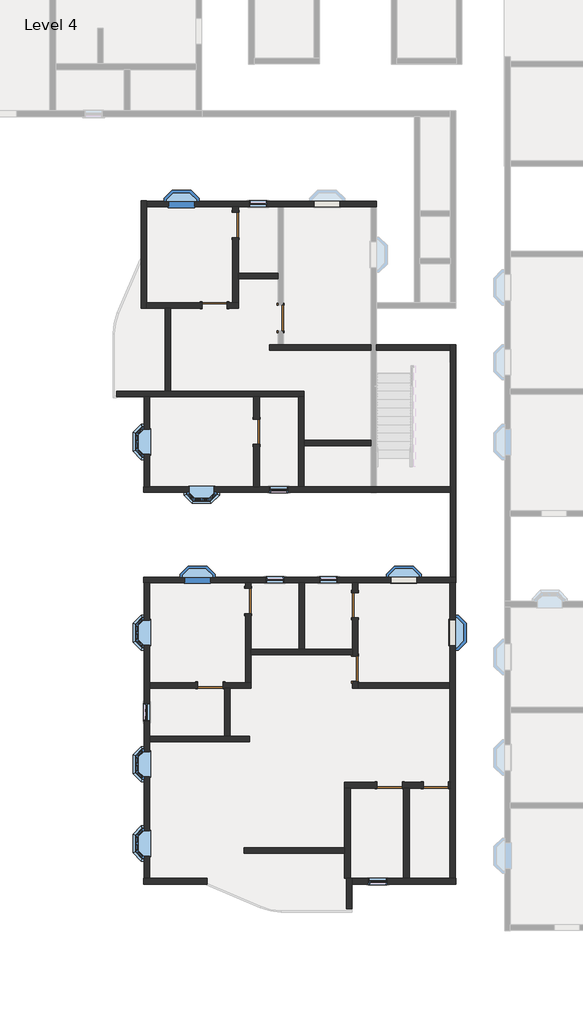
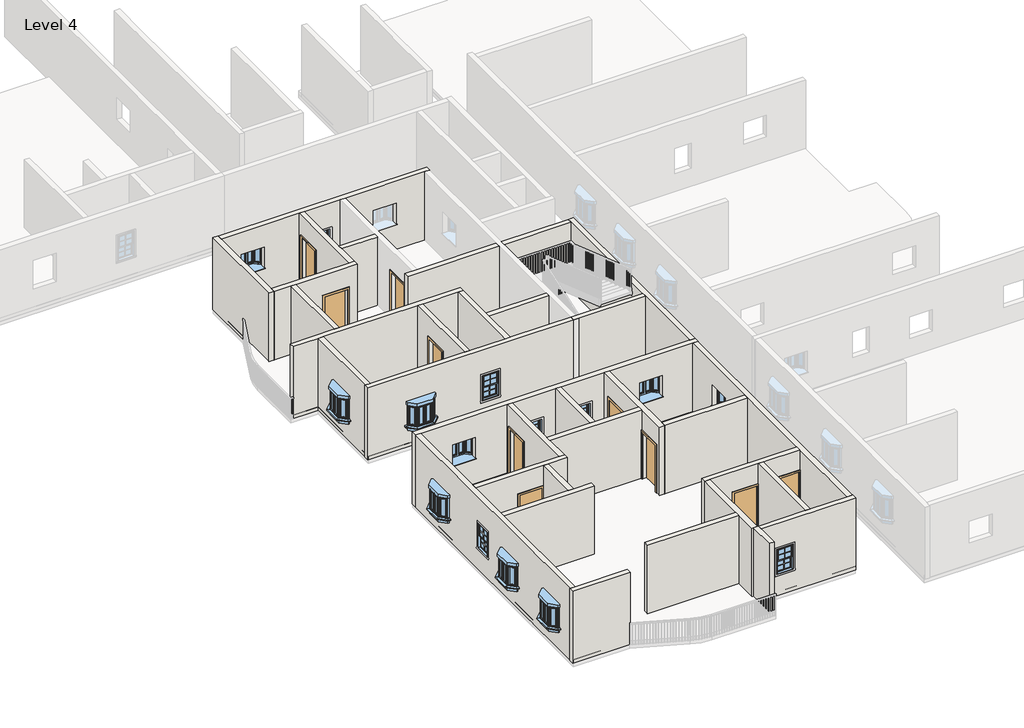
# One storey, part 1 of 14: 32 walls, 15 windows, 10 doors.
"""IFC4 building model written with IfcOpenShell, lengths in millimetres."""

from ifc_helpers import new_model, si_unit, frame, origin, place, context, project, spatial, polyline, outline, extrude, faceted_brep, transform, mapped, element, save
from components import door_54dd4da4, door_719f80de, window_910x910mm_67ef725a, window_8debb0fa

model = new_model("IFC4")

# Units and contexts
model_context = context("Model", 3, world=origin())
ifc_project = project(units=[si_unit("LENGTHUNIT", "METRE", prefix="MILLI")], contexts=[model_context])

# Site, building, storey
site = spatial("IfcSite", under=ifc_project)
building = spatial("IfcBuilding", under=site)
storey = spatial("IfcBuildingStorey", under=building, Name="Level 4", Elevation=9144.0)

# Doors
placement = place(None, origin())
door_shape = door_54dd4da4(model_context)
element("IfcDoor", 1, ObjectType="Single-Flush : 36\" x 84\"", at=placement, inside=storey, context=model_context, shape_type="MappedRepresentation", body=[
    mapped(door_shape, transform((-4626.037215, -17283.4916506, 9144.0), x_axis=(0.0, -1.0, 0.0), y_axis=(1.0, 0.0, 0.0), z_axis=(0.0, 0.0, 1.0))),
])
element("IfcDoor", 2, ObjectType="Single-Flush : 36\" x 84\"", at=placement, inside=storey, context=model_context, shape_type="MappedRepresentation", body=[
    mapped(door_shape, transform((-4626.037215, -14978.4416506, 9144.0), x_axis=(0.0, 1.0, 0.0), y_axis=(-1.0, 0.0, 0.0), z_axis=(0.0, 0.0, 1.0))),
])
element("IfcDoor", 3, ObjectType="Single-Flush : 36\" x 84\"", at=placement, inside=storey, context=model_context, shape_type="MappedRepresentation", body=[
    mapped(door_shape, transform((-9731.437215, -4100.8916506, 9144.0), x_axis=(1.0, 0.0, 0.0), y_axis=(0.0, 1.0, 0.0), z_axis=(0.0, 0.0, 1.0))),
])
element("IfcDoor", 4, ObjectType="Single-Flush : 36\" x 84\"", at=placement, inside=storey, context=model_context, shape_type="MappedRepresentation", body=[
    mapped(door_shape, transform((-7331.137215, -4558.0916506, 9144.0), x_axis=(0.0, -1.0, 0.0), y_axis=(1.0, 0.0, 0.0), z_axis=(0.0, 0.0, 1.0))),
])
door_2_shape = door_719f80de(model_context)
element("IfcDoor", 5, ObjectType="Single-Flush : 36\" x 84\"", at=placement, inside=storey, context=model_context, shape_type="MappedRepresentation", body=[
    mapped(door_2_shape, transform((-9883.837215, -17891.2072331, 9144.0), x_axis=(1.0, 0.0, 0.0), y_axis=(0.0, 1.0, 0.0), z_axis=(0.0, 0.0, 1.0))),
])
element("IfcDoor", 6, ObjectType="Single-Flush : 36\" x 84\"", at=placement, inside=storey, context=model_context, shape_type="MappedRepresentation", body=[
    mapped(door_2_shape, transform((-8512.237215, -14826.0416506, 9144.0), x_axis=(0.0, 1.0, 0.0), y_axis=(-1.0, 0.0, 0.0), z_axis=(0.0, 0.0, 1.0))),
])
element("IfcDoor", 7, ObjectType="Single-Flush : 36\" x 84\"", at=placement, inside=storey, context=model_context, shape_type="MappedRepresentation", body=[
    mapped(door_2_shape, transform((-8207.437215, -8691.9416506, 9144.0), x_axis=(0.0, 1.0, 0.0), y_axis=(-1.0, 0.0, 0.0), z_axis=(0.0, 0.0, 1.0))),
])
element("IfcDoor", 8, ObjectType="Single-Flush : 36\" x 84\"", at=placement, inside=storey, context=model_context, shape_type="MappedRepresentation", body=[
    mapped(door_2_shape, transform((-8969.437215, -1186.2416506, 9144.0), x_axis=(0.0, 1.0, 0.0), y_axis=(-1.0, 0.0, 0.0), z_axis=(0.0, 0.0, 1.0))),
])
element("IfcDoor", 9, ObjectType="Single-Flush : 36\" x 84\"", at=placement, inside=storey, context=model_context, shape_type="MappedRepresentation", body=[
    mapped(door_2_shape, transform((-3374.4891351, -21512.5916506, 9144.0), x_axis=(1.0, 0.0, 0.0), y_axis=(0.0, 1.0, 0.0), z_axis=(0.0, 0.0, 1.0))),
])
element("IfcDoor", 10, ObjectType="Single-Flush : 36\" x 84\"", at=placement, inside=storey, context=model_context, shape_type="MappedRepresentation", body=[
    mapped(door_2_shape, transform((-1698.0891351, -21512.5916506, 9144.0), x_axis=(1.0, 0.0, 0.0), y_axis=(0.0, 1.0, 0.0), z_axis=(0.0, 0.0, 1.0))),
])

# Walls
element("IfcWall", 11, ObjectType="4.5\" p", at=placement, inside=storey, context=model_context, shape_type="Brep", body=[
    faceted_brep([(-9426.637215, -17992.8072331, 11277.6), (-9426.637215, -17992.8072331, 9144.0), (-9375.837215, -17992.8072331, 9144.0), (-9172.637215, -17992.8072331, 9144.0), (-8410.637215, -17992.8072331, 9144.0), (-8410.637215, -17992.8072331, 12192.0), (-9172.637215, -17992.8072331, 12192.0), (-9375.837215, -17992.8072331, 12192.0), (-12087.287215, -17992.8072331, 12192.0), (-12087.287215, -17992.8072331, 9144.0), (-10341.037215, -17992.8072331, 9144.0), (-10341.037215, -17992.8072331, 11277.6), (-8410.637215, -17789.6072331, 9144.0), (-8613.837215, -17789.6072331, 9144.0), (-9426.637215, -17789.6072331, 9144.0), (-9426.637215, -17789.6072331, 11277.6), (-10341.037215, -17789.6072331, 11277.6), (-10341.037215, -17789.6072331, 9144.0), (-12087.287215, -17789.6072331, 9144.0), (-12087.287215, -17789.6072331, 12192.0), (-8613.837215, -17789.6072331, 12192.0), (-8410.637215, -17789.6072331, 12192.0)], [[[0, 1, 2, 3, 4, 5, 6, 7, 8, 9, 10, 11]], [[12, 13, 14, 15, 16, 17, 18, 19, 20, 21]], [[10, 9, 18, 17]], [[4, 3, 2, 1, 14, 13, 12]], [[8, 7, 6, 5, 21, 20, 19]], [[9, 8, 19, 18]], [[5, 4, 12, 21]], [[15, 14, 1, 0]], [[16, 15, 0, 11]], [[17, 16, 11, 10]]]),
])
element("IfcWall", 12, ObjectType="4.5\" p", at=placement, inside=storey, context=model_context, shape_type="Brep", body=[
    faceted_brep([(-8410.637215, -14368.8416506, 11277.6), (-8410.637215, -14368.8416506, 9144.0), (-8410.637215, -14165.6416506, 9144.0), (-8410.637215, -14165.6416506, 12192.0), (-8410.637215, -16572.2916506, 12192.0), (-8410.637215, -16775.4916506, 12192.0), (-8410.637215, -17789.6072331, 12192.0), (-8410.637215, -17789.6072331, 9144.0), (-8410.637215, -16775.4916506, 9144.0), (-8410.637215, -16572.2916506, 9144.0), (-8410.637215, -15283.2416506, 9144.0), (-8410.637215, -15283.2416506, 11277.6), (-8613.837215, -14165.6416506, 9144.0), (-8613.837215, -14368.8416506, 9144.0), (-8613.837215, -14368.8416506, 11277.6), (-8613.837215, -15283.2416506, 11277.6), (-8613.837215, -15283.2416506, 9144.0), (-8613.837215, -17789.6072331, 9144.0), (-8613.837215, -17789.6072331, 12192.0), (-8613.837215, -14165.6416506, 12192.0)], [[[0, 1, 2, 3, 4, 5, 6, 7, 8, 9, 10, 11]], [[12, 13, 14, 15, 16, 17, 18, 19]], [[2, 1, 13, 12]], [[10, 9, 8, 7, 17, 16]], [[6, 5, 4, 3, 19, 18]], [[7, 6, 18, 17]], [[3, 2, 12, 19]], [[14, 13, 1, 0]], [[15, 14, 0, 11]], [[16, 15, 11, 10]]]),
])
element("IfcWall", 13, ObjectType="4.5\" p", at=placement, inside=storey, context=model_context, shape_type="Brep", body=[
    faceted_brep([(-8410.637215, -16775.4916506, 9144.0), (-4727.637215, -16775.4916506, 9144.0), (-4727.637215, -16775.4916506, 12192.0), (-8410.637215, -16775.4916506, 12192.0), (-8410.637215, -16572.2916506, 9144.0), (-8410.637215, -16572.2916506, 12192.0), (-6670.737215, -16572.2916506, 12192.0), (-6467.537215, -16572.2916506, 12192.0), (-4727.637215, -16572.2916506, 12192.0), (-4727.637215, -16572.2916506, 9144.0), (-6467.537215, -16572.2916506, 9144.0), (-6670.737215, -16572.2916506, 9144.0)], [[[0, 1, 2, 3]], [[4, 5, 6, 7, 8, 9, 10, 11]], [[1, 0, 4, 11, 10, 9]], [[3, 2, 8, 7, 6, 5]], [[0, 3, 5, 4]], [[2, 1, 9, 8]]]),
])
element("IfcWall", 14, ObjectType="4.5\" p", at=placement, inside=storey, context=model_context, shape_type="SweptSolid", body=[
    extrude(outline(polyline([(-6670.737215, -16572.2916506), (-6670.737215, -14165.6416506), (-6467.537215, -14165.6416506), (-6467.537215, -16572.2916506), (-6670.737215, -16572.2916506)])), frame((0.0, 0.0, 9144.0), z_axis=(0.0, 0.0, 1.0), x_axis=(1.0, 0.0, 0.0)), (0.0, 0.0, 1.0), 3048.0),
])
element("IfcWall", 15, ObjectType="4.5\" p", at=placement, inside=storey, context=model_context, shape_type="Brep", body=[
    faceted_brep([(-4727.637215, -14165.6416506, 9144.0), (-4727.637215, -14521.2416506, 9144.0), (-4727.637215, -14521.2416506, 11277.6), (-4727.637215, -15435.6416506, 11277.6), (-4727.637215, -15435.6416506, 9144.0), (-4727.637215, -16572.2916506, 9144.0), (-4727.637215, -16775.4916506, 9144.0), (-4727.637215, -16826.2916506, 9144.0), (-4727.637215, -16826.2916506, 11277.6), (-4727.637215, -17740.6916506, 11277.6), (-4727.637215, -17740.6916506, 9144.0), (-4727.637215, -17994.6916506, 9144.0), (-4727.637215, -17994.6916506, 12192.0), (-4727.637215, -16775.4916506, 12192.0), (-4727.637215, -16572.2916506, 12192.0), (-4727.637215, -14165.6416506, 12192.0), (-4524.437215, -14521.2416506, 11277.6), (-4524.437215, -14521.2416506, 9144.0), (-4524.437215, -14165.6416506, 9144.0), (-4524.437215, -14165.6416506, 12192.0), (-4524.437215, -17791.4916506, 12192.0), (-4524.437215, -17994.6916506, 12192.0), (-4524.437215, -17994.6916506, 9144.0), (-4524.437215, -17791.4916506, 9144.0), (-4524.437215, -17740.6916506, 9144.0), (-4524.437215, -17740.6916506, 11277.6), (-4524.437215, -16826.2916506, 11277.6), (-4524.437215, -16826.2916506, 9144.0), (-4524.437215, -15435.6416506, 9144.0), (-4524.437215, -15435.6416506, 11277.6)], [[[0, 1, 2, 3, 4, 5, 6, 7, 8, 9, 10, 11, 12, 13, 14, 15]], [[16, 17, 18, 19, 20, 21, 22, 23, 24, 25, 26, 27, 28, 29]], [[11, 10, 24, 23, 22]], [[28, 27, 7, 6, 5, 4]], [[18, 17, 1, 0]], [[15, 14, 13, 12, 21, 20, 19]], [[0, 15, 19, 18]], [[12, 11, 22, 21]], [[25, 24, 10, 9]], [[26, 25, 9, 8]], [[27, 26, 8, 7]], [[2, 1, 17, 16]], [[3, 2, 16, 29]], [[4, 3, 29, 28]]]),
])
element("IfcWall", 16, ObjectType="4.5\" p", at=placement, inside=storey, context=model_context, shape_type="SweptSolid", body=[
    extrude(outline(polyline([(-4524.437215, -17791.4916506), (-1190.0891351, -17791.4916506), (-1190.0891351, -17994.6916506), (-4524.437215, -17994.6916506), (-4524.437215, -17791.4916506)])), frame((0.0, 0.0, 9144.0), z_axis=(0.0, 0.0, 1.0), x_axis=(1.0, 0.0, 0.0)), (0.0, 0.0, 1.0), 3048.0),
])
element("IfcWall", 17, ObjectType="4.5\" p", at=placement, inside=storey, context=model_context, shape_type="SweptSolid", body=[
    extrude(outline(polyline([(-9375.837215, -19734.5916506), (-9375.837215, -17992.8072331), (-9172.637215, -17992.8072331), (-9172.637215, -19734.5916506), (-9375.837215, -19734.5916506)])), frame((0.0, 0.0, 9144.0), z_axis=(0.0, 0.0, 1.0), x_axis=(1.0, 0.0, 0.0)), (0.0, 0.0, 1.0), 3048.0),
])
element("IfcWall", 18, ObjectType="4.5\" p", at=placement, inside=storey, context=model_context, shape_type="Brep", body=[
    faceted_brep([(-12087.287215, -19937.7916506, 9144.0), (-8455.087215, -19937.7916506, 9144.0), (-8455.087215, -19937.7916506, 12192.0), (-12087.287215, -19937.7916506, 12192.0), (-12087.287215, -19734.5916506, 9144.0), (-12087.287215, -19734.5916506, 12192.0), (-9375.837215, -19734.5916506, 12192.0), (-9172.637215, -19734.5916506, 12192.0), (-8455.087215, -19734.5916506, 12192.0), (-8455.087215, -19734.5916506, 9144.0), (-9172.637215, -19734.5916506, 9144.0), (-9375.837215, -19734.5916506, 9144.0)], [[[0, 1, 2, 3]], [[4, 5, 6, 7, 8, 9, 10, 11]], [[1, 0, 4, 11, 10, 9]], [[2, 1, 9, 8]], [[3, 2, 8, 7, 6, 5]], [[0, 3, 5, 4]]]),
])
element("IfcWall", 19, ObjectType="4.5\" p", at=placement, inside=storey, context=model_context, shape_type="Brep", body=[
    faceted_brep([(-13293.787215, -7421.9416506, 9144.0), (-12290.487215, -7421.9416506, 9144.0), (-12087.287215, -7421.9416506, 9144.0), (-8309.037215, -7421.9416506, 9144.0), (-8105.837215, -7421.9416506, 9144.0), (-6689.787215, -7421.9416506, 9144.0), (-6486.587215, -7421.9416506, 9144.0), (-6486.587215, -7421.9416506, 12192.0), (-6689.787215, -7421.9416506, 12192.0), (-8105.837215, -7421.9416506, 12192.0), (-8309.037215, -7421.9416506, 12192.0), (-12087.287215, -7421.9416506, 12192.0), (-12290.487215, -7421.9416506, 12192.0), (-13293.787215, -7421.9416506, 12192.0), (-13293.787215, -7218.7416506, 9144.0), (-13293.787215, -7218.7416506, 12192.0), (-11528.487215, -7218.7416506, 12192.0), (-11325.287215, -7218.7416506, 12192.0), (-6486.587215, -7218.7416506, 12192.0), (-6486.587215, -7218.7416506, 9144.0), (-11325.287215, -7218.7416506, 9144.0), (-11528.487215, -7218.7416506, 9144.0)], [[[0, 1, 2, 3, 4, 5, 6, 7, 8, 9, 10, 11, 12, 13]], [[14, 15, 16, 17, 18, 19, 20, 21]], [[6, 5, 4, 3, 2, 1, 0, 14, 21, 20, 19]], [[13, 12, 11, 10, 9, 8, 7, 18, 17, 16, 15]], [[0, 13, 15, 14]], [[7, 6, 19, 18]]]),
])
element("IfcWall", 20, ObjectType="4.5\" p", at=placement, inside=storey, context=model_context, shape_type="Brep", body=[
    faceted_brep([(-12201.587215, -4202.4916506, 9144.0), (-12201.587215, -3999.2916506, 9144.0), (-12201.587215, -525.8416506, 9144.0), (-12201.587215, -322.6416506, 9144.0), (-12201.587215, -309.9416506, 9144.0), (-12201.587215, -309.9416506, 12192.0), (-12201.587215, -322.6416506, 12192.0), (-12201.587215, -525.8416506, 12192.0), (-12201.587215, -3999.2916506, 12192.0), (-12201.587215, -4202.4916506, 12192.0), (-12404.787215, -4202.4916506, 9144.0), (-12404.787215, -4202.4916506, 12192.0), (-12404.787215, -309.9416506, 12192.0), (-12404.787215, -309.9416506, 9144.0)], [[[0, 1, 2, 3, 4, 5, 6, 7, 8, 9]], [[10, 11, 12, 13]], [[4, 3, 2, 1, 0, 10, 13]], [[5, 4, 13, 12]], [[9, 8, 7, 6, 5, 12, 11]], [[0, 9, 11, 10]]]),
])
element("IfcWall", 21, ObjectType="4.5\" p", at=placement, inside=storey, context=model_context, shape_type="Brep", body=[
    faceted_brep([(-9274.237215, -4202.4916506, 11277.6), (-9274.237215, -4202.4916506, 9144.0), (-8867.837215, -4202.4916506, 9144.0), (-8867.837215, -4202.4916506, 12192.0), (-11325.287215, -4202.4916506, 12192.0), (-11528.487215, -4202.4916506, 12192.0), (-12201.587215, -4202.4916506, 12192.0), (-12201.587215, -4202.4916506, 9144.0), (-11528.487215, -4202.4916506, 9144.0), (-11325.287215, -4202.4916506, 9144.0), (-10188.637215, -4202.4916506, 9144.0), (-10188.637215, -4202.4916506, 11277.6), (-8867.837215, -3999.2916506, 9144.0), (-9071.037215, -3999.2916506, 9144.0), (-9274.237215, -3999.2916506, 9144.0), (-9274.237215, -3999.2916506, 11277.6), (-10188.637215, -3999.2916506, 11277.6), (-10188.637215, -3999.2916506, 9144.0), (-12201.587215, -3999.2916506, 9144.0), (-12201.587215, -3999.2916506, 12192.0), (-9071.037215, -3999.2916506, 12192.0), (-8867.837215, -3999.2916506, 12192.0)], [[[0, 1, 2, 3, 4, 5, 6, 7, 8, 9, 10, 11]], [[12, 13, 14, 15, 16, 17, 18, 19, 20, 21]], [[2, 1, 14, 13, 12]], [[10, 9, 8, 7, 18, 17]], [[6, 5, 4, 3, 21, 20, 19]], [[7, 6, 19, 18]], [[3, 2, 12, 21]], [[15, 14, 1, 0]], [[16, 15, 0, 11]], [[17, 16, 11, 10]]]),
])
element("IfcWall", 22, ObjectType="4.5\" p", at=placement, inside=storey, context=model_context, shape_type="Brep", body=[
    faceted_brep([(-8867.837215, -729.0416506, 11277.6), (-8867.837215, -729.0416506, 9144.0), (-8867.837215, -525.8416506, 9144.0), (-8867.837215, -525.8416506, 12192.0), (-8867.837215, -2932.4916506, 12192.0), (-8867.837215, -3135.6916506, 12192.0), (-8867.837215, -3999.2916506, 12192.0), (-8867.837215, -3999.2916506, 9144.0), (-8867.837215, -3135.6916506, 9144.0), (-8867.837215, -2932.4916506, 9144.0), (-8867.837215, -1643.4416506, 9144.0), (-8867.837215, -1643.4416506, 11277.6), (-9071.037215, -525.8416506, 9144.0), (-9071.037215, -729.0416506, 9144.0), (-9071.037215, -729.0416506, 11277.6), (-9071.037215, -1643.4416506, 11277.6), (-9071.037215, -1643.4416506, 9144.0), (-9071.037215, -3999.2916506, 9144.0), (-9071.037215, -3999.2916506, 12192.0), (-9071.037215, -525.8416506, 12192.0)], [[[0, 1, 2, 3, 4, 5, 6, 7, 8, 9, 10, 11]], [[12, 13, 14, 15, 16, 17, 18, 19]], [[2, 1, 13, 12]], [[10, 9, 8, 7, 17, 16]], [[6, 5, 4, 3, 19, 18]], [[7, 6, 18, 17]], [[3, 2, 12, 19]], [[14, 13, 1, 0]], [[15, 14, 0, 11]], [[16, 15, 11, 10]]]),
])
element("IfcWall", 23, ObjectType="4.5\" p", at=placement, inside=storey, context=model_context, shape_type="SweptSolid", body=[
    extrude(outline(polyline([(-7432.737215, -3135.6916506), (-8867.837215, -3135.6916506), (-8867.837215, -2932.4916506), (-7432.737215, -2932.4916506), (-7432.737215, -3135.6916506)])), frame((0.0, 0.0, 9144.0), z_axis=(0.0, 0.0, 1.0), x_axis=(1.0, 0.0, 0.0)), (0.0, 0.0, 1.0), 3048.0),
])
element("IfcWall", 24, ObjectType="4.5\" p", at=placement, inside=storey, context=model_context, shape_type="Brep", body=[
    faceted_brep([(-7731.187215, -5726.4916506, 12192.0), (-7731.187215, -5726.4916506, 9144.0), (-4060.887215, -5726.4916506, 9144.0), (-4060.887215, -5726.4916506, 12192.0), (-7731.187215, -5523.2916506, 9144.0), (-7731.187215, -5523.2916506, 12192.0), (-7432.737215, -5523.2916506, 12192.0), (-7229.537215, -5523.2916506, 12192.0), (-4060.887215, -5523.2916506, 12192.0), (-4060.887215, -5523.2916506, 9144.0), (-7229.537215, -5523.2916506, 9144.0), (-7432.737215, -5523.2916506, 9144.0)], [[[0, 1, 2, 3]], [[4, 5, 6, 7, 8, 9, 10, 11]], [[1, 4, 11, 10, 9, 2]], [[5, 0, 3, 8, 7, 6]], [[1, 0, 5, 4]], [[3, 2, 9, 8]]]),
    faceted_brep([(-1177.3891351, -5726.4916506, 9144.0), (-1177.3891351, -5726.4916506, 12192.0), (-3857.687215, -5726.4916506, 12192.0), (-3857.687215, -5726.4916506, 9144.0), (-1177.3891351, -5523.2916506, 12192.0), (-1177.3891351, -5523.2916506, 9144.0), (-3857.687215, -5523.2916506, 9144.0), (-3857.687215, -5523.2916506, 12192.0)], [[[0, 1, 2, 3]], [[4, 5, 6, 7]], [[5, 0, 3, 6]], [[1, 4, 7, 2]], [[1, 0, 5, 4]], [[3, 2, 7, 6]]]),
])
element("IfcWall", 25, ObjectType="4.5\" p", at=placement, inside=storey, context=model_context, shape_type="SweptSolid", body=[
    extrude(outline(polyline([(-11528.487215, -7218.7416506), (-11528.487215, -4202.4916506), (-11325.287215, -4202.4916506), (-11325.287215, -7218.7416506), (-11528.487215, -7218.7416506)])), frame((0.0, 0.0, 9144.0), z_axis=(0.0, 0.0, 1.0), x_axis=(1.0, 0.0, 0.0)), (0.0, 0.0, 1.0), 3048.0),
])
element("IfcWall", 26, ObjectType="4.5\" p", at=placement, inside=storey, context=model_context, shape_type="SweptSolid", body=[
    extrude(outline(polyline([(-7421.9416506, 9144.0), (-8234.7416506, 9144.0), (-8234.7416506, 11277.6), (-9149.1416506, 11277.6), (-9149.1416506, 9144.0), (-10685.8416506, 9144.0), (-10685.8416506, 12192.0), (-7421.9416506, 12192.0), (-7421.9416506, 9144.0)])), frame((-8309.037215, 0.0, 0.0), z_axis=(1.0, 0.0, 0.0), x_axis=(0.0, 1.0, 0.0)), (0.0, 0.0, 1.0), 203.2),
])
element("IfcWall", 27, ObjectType="4.5\" p", at=placement, inside=storey, context=model_context, shape_type="Brep", body=[
    faceted_brep([(-6689.787215, -7421.9416506, 9144.0), (-6689.787215, -10685.8416506, 9144.0), (-6689.787215, -10685.8416506, 12192.0), (-6689.787215, -7421.9416506, 12192.0), (-6486.587215, -7421.9416506, 9144.0), (-6486.587215, -7421.9416506, 12192.0), (-6486.587215, -8990.3916506, 12192.0), (-6486.587215, -9193.5916506, 12192.0), (-6486.587215, -10685.8416506, 12192.0), (-6486.587215, -10685.8416506, 9144.0), (-6486.587215, -9193.5916506, 9144.0), (-6486.587215, -8990.3916506, 9144.0)], [[[0, 1, 2, 3]], [[4, 5, 6, 7, 8, 9, 10, 11]], [[1, 0, 4, 11, 10, 9]], [[3, 2, 8, 7, 6, 5]], [[0, 3, 5, 4]], [[2, 1, 9, 8]]]),
])
element("IfcWall", 28, ObjectType="4.5\" p", at=placement, inside=storey, context=model_context, shape_type="SweptSolid", body=[
    extrude(outline(polyline([(-4060.887215, -9193.5916506), (-6486.587215, -9193.5916506), (-6486.587215, -8990.3916506), (-4060.887215, -8990.3916506), (-4060.887215, -9193.5916506)])), frame((0.0, 0.0, 9144.0), z_axis=(0.0, 0.0, 1.0), x_axis=(1.0, 0.0, 0.0)), (0.0, 0.0, 1.0), 3048.0),
])
element("IfcWall", 29, ObjectType="9\"", at=placement, inside=storey, context=model_context, shape_type="Brep", body=[
    faceted_brep([(-1190.0891351, -21410.9916506, 9144.0), (-1240.8891351, -21410.9916506, 9144.0), (-1240.8891351, -21410.9916506, 11277.6), (-2155.2891351, -21410.9916506, 11277.6), (-2155.2891351, -21410.9916506, 9144.0), (-2917.2891351, -21410.9916506, 9144.0), (-2917.2891351, -21410.9916506, 11277.6), (-3831.6891351, -21410.9916506, 11277.6), (-3831.6891351, -21410.9916506, 9144.0), (-5006.4391351, -21410.9916506, 9144.0), (-5006.4391351, -21410.9916506, 12192.0), (-1190.0891351, -21410.9916506, 12192.0), (-1240.8891351, -21614.1916506, 11277.6), (-1240.8891351, -21614.1916506, 9144.0), (-1190.0891351, -21614.1916506, 9144.0), (-1190.0891351, -21614.1916506, 12192.0), (-2663.2891351, -21614.1916506, 12192.0), (-2866.4891351, -21614.1916506, 12192.0), (-4803.2391351, -21614.1916506, 12192.0), (-5006.4391351, -21614.1916506, 12192.0), (-5006.4391351, -21614.1916506, 9144.0), (-4803.2391351, -21614.1916506, 9144.0), (-3831.6891351, -21614.1916506, 9144.0), (-3831.6891351, -21614.1916506, 11277.6), (-2917.2891351, -21614.1916506, 11277.6), (-2917.2891351, -21614.1916506, 9144.0), (-2866.4891351, -21614.1916506, 9144.0), (-2663.2891351, -21614.1916506, 9144.0), (-2155.2891351, -21614.1916506, 9144.0), (-2155.2891351, -21614.1916506, 11277.6)], [[[0, 1, 2, 3, 4, 5, 6, 7, 8, 9, 10, 11]], [[12, 13, 14, 15, 16, 17, 18, 19, 20, 21, 22, 23, 24, 25, 26, 27, 28, 29]], [[22, 21, 20, 9, 8]], [[14, 13, 1, 0]], [[28, 27, 26, 25, 5, 4]], [[11, 10, 19, 18, 17, 16, 15]], [[0, 11, 15, 14]], [[10, 9, 20, 19]], [[6, 5, 25, 24]], [[7, 6, 24, 23]], [[8, 7, 23, 22]], [[2, 1, 13, 12]], [[3, 2, 12, 29]], [[4, 3, 29, 28]]]),
])
element("IfcWall", 30, ObjectType="9\"", at=placement, inside=storey, context=model_context, shape_type="Brep", body=[
    faceted_brep([(-5006.4391351, -21614.1916506, 9144.0), (-5006.4391351, -23779.5416506, 9144.0), (-5006.4391351, -23982.7416506, 9144.0), (-5006.4391351, -24897.1416506, 9144.0), (-5006.4391351, -24897.1416506, 12192.0), (-5006.4391351, -23982.7416506, 12192.0), (-5006.4391351, -23779.5416506, 12192.0), (-5006.4391351, -21614.1916506, 12192.0), (-4803.2391351, -21614.1916506, 9144.0), (-4803.2391351, -21614.1916506, 12192.0), (-4803.2391351, -24897.1416506, 12192.0), (-4803.2391351, -24897.1416506, 9144.0), (-4949.2891351, -24897.1416506, 9144.0), (-4949.2891351, -24897.1416506, 12192.0)], [[[0, 1, 2, 3, 4, 5, 6, 7]], [[8, 9, 10, 11]], [[3, 2, 1, 0, 8, 11, 12]], [[7, 6, 5, 4, 13, 10, 9]], [[0, 7, 9, 8]], [[4, 3, 12, 11, 10, 13]]]),
])
element("IfcWall", 31, ObjectType="9\"", at=placement, inside=storey, context=model_context, shape_type="SweptSolid", body=[
    extrude(outline(polyline([(-2866.4891351, -24897.1416506), (-2866.4891351, -21614.1916506), (-2663.2891351, -21614.1916506), (-2663.2891351, -24897.1416506), (-2866.4891351, -24897.1416506)])), frame((0.0, 0.0, 9144.0), z_axis=(0.0, 0.0, 1.0), x_axis=(1.0, 0.0, 0.0)), (0.0, 0.0, 1.0), 3048.0),
])
element("IfcWall", 32, ObjectType="9\"", at=placement, inside=storey, context=model_context, shape_type="SweptSolid", body=[
    extrude(outline(polyline([(-5006.4391351, -23982.7416506), (-8664.637215, -23982.7416506), (-8664.637215, -23779.5416506), (-5006.4391351, -23779.5416506), (-5006.4391351, -23982.7416506)])), frame((0.0, 0.0, 9144.0), z_axis=(0.0, 0.0, 1.0), x_axis=(1.0, 0.0, 0.0)), (0.0, 0.0, 1.0), 3048.0),
])
element("IfcWall", 33, ObjectType="9\" w", at=placement, inside=storey, context=model_context, shape_type="Brep", body=[
    faceted_brep([(-12303.187215, -14165.6416506, 9144.0), (-12290.487215, -14165.6416506, 9144.0), (-12087.287215, -14165.6416506, 9144.0), (-8613.837215, -14165.6416506, 9144.0), (-8410.637215, -14165.6416506, 9144.0), (-6670.737215, -14165.6416506, 9144.0), (-6467.537215, -14165.6416506, 9144.0), (-4727.637215, -14165.6416506, 9144.0), (-4524.437215, -14165.6416506, 9144.0), (-1190.0891351, -14165.6416506, 9144.0), (-986.8891351, -14165.6416506, 9144.0), (-961.4891351, -14165.6416506, 9144.0), (-961.4891351, -14165.6416506, 12192.0), (-986.8891351, -14165.6416506, 12192.0), (-1190.0891351, -14165.6416506, 12192.0), (-4524.437215, -14165.6416506, 12192.0), (-4727.637215, -14165.6416506, 12192.0), (-6467.537215, -14165.6416506, 12192.0), (-6670.737215, -14165.6416506, 12192.0), (-8410.637215, -14165.6416506, 12192.0), (-8613.837215, -14165.6416506, 12192.0), (-12087.287215, -14165.6416506, 12192.0), (-12290.487215, -14165.6416506, 12192.0), (-12303.187215, -14165.6416506, 12192.0), (-10805.562215, -14165.6416506, 11254.0), (-9895.562215, -14165.6416506, 11254.0), (-9895.562215, -14165.6416506, 10344.0), (-10805.562215, -14165.6416506, 10344.0), (-3312.2631751, -14165.6416506, 11254.0), (-2402.2631751, -14165.6416506, 11254.0), (-2402.2631751, -14165.6416506, 10344.0), (-3312.2631751, -14165.6416506, 10344.0), (-7870.887215, -14165.6416506, 11125.2), (-7210.487215, -14165.6416506, 11125.2), (-7210.487215, -14165.6416506, 10058.4), (-7870.887215, -14165.6416506, 10058.4), (-5927.787215, -14165.6416506, 11125.2), (-5267.387215, -14165.6416506, 11125.2), (-5267.387215, -14165.6416506, 10058.4), (-5927.787215, -14165.6416506, 10058.4), (-12303.187215, -13962.4416506, 9144.0), (-12303.187215, -13962.4416506, 12192.0), (-1177.3891351, -13962.4416506, 12192.0), (-974.1891351, -13962.4416506, 12192.0), (-961.4891351, -13962.4416506, 12192.0), (-961.4891351, -13962.4416506, 9144.0), (-974.1891351, -13962.4416506, 9144.0), (-1177.3891351, -13962.4416506, 9144.0), (-10805.562215, -13962.4416506, 11254.0), (-10805.562215, -13962.4416506, 10344.0), (-9895.562215, -13962.4416506, 10344.0), (-9895.562215, -13962.4416506, 11254.0), (-3312.2631751, -13962.4416506, 11254.0), (-3312.2631751, -13962.4416506, 10344.0), (-2402.2631751, -13962.4416506, 10344.0), (-2402.2631751, -13962.4416506, 11254.0), (-7870.887215, -13962.4416506, 11125.2), (-7870.887215, -13962.4416506, 10058.4), (-7210.487215, -13962.4416506, 10058.4), (-7210.487215, -13962.4416506, 11125.2), (-5927.787215, -13962.4416506, 11125.2), (-5927.787215, -13962.4416506, 10058.4), (-5267.387215, -13962.4416506, 10058.4), (-5267.387215, -13962.4416506, 11125.2)], [[[0, 1, 2, 3, 4, 5, 6, 7, 8, 9, 10, 11, 12, 13, 14, 15, 16, 17, 18, 19, 20, 21, 22, 23], [24, 25, 26, 27], [28, 29, 30, 31], [32, 33, 34, 35], [36, 37, 38, 39]], [[40, 41, 42, 43, 44, 45, 46, 47], [48, 49, 50, 51], [52, 53, 54, 55], [56, 57, 58, 59], [60, 61, 62, 63]], [[11, 10, 9, 8, 7, 6, 5, 4, 3, 2, 1, 0, 40, 47, 46, 45]], [[12, 11, 45, 44]], [[23, 22, 21, 20, 19, 18, 17, 16, 15, 14, 13, 12, 44, 43, 42, 41]], [[0, 23, 41, 40]], [[49, 48, 24, 27]], [[50, 49, 27, 26]], [[51, 50, 26, 25]], [[48, 51, 25, 24]], [[53, 52, 28, 31]], [[54, 53, 31, 30]], [[55, 54, 30, 29]], [[52, 55, 29, 28]], [[57, 56, 32, 35]], [[58, 57, 35, 34]], [[59, 58, 34, 33]], [[56, 59, 33, 32]], [[61, 60, 36, 39]], [[62, 61, 39, 38]], [[63, 62, 38, 37]], [[60, 63, 37, 36]]]),
])
element("IfcWall", 34, ObjectType="9\" w", at=placement, inside=storey, context=model_context, shape_type="Brep", body=[
    faceted_brep([(-10004.0323936, -24897.1416506, 9144.0), (-12087.287215, -24897.1416506, 9144.0), (-12290.487215, -24897.1416506, 9144.0), (-12303.187215, -24897.1416506, 9144.0), (-12303.187215, -24897.1416506, 12192.0), (-12290.487215, -24897.1416506, 12192.0), (-12087.287215, -24897.1416506, 12192.0), (-10004.0323936, -24897.1416506, 12192.0), (-10004.0323936, -25100.3416506, 9144.0), (-10004.0323936, -25100.3416506, 12192.0), (-12303.187215, -25100.3416506, 12192.0), (-12303.187215, -25100.3416506, 9144.0)], [[[0, 1, 2, 3, 4, 5, 6, 7]], [[8, 9, 10, 11]], [[3, 2, 1, 0, 8, 11]], [[4, 3, 11, 10]], [[7, 6, 5, 4, 10, 9]], [[0, 7, 9, 8]]]),
])
element("IfcWall", 35, ObjectType="9\" w", at=placement, inside=storey, context=model_context, shape_type="Brep", body=[
    faceted_brep([(-4746.0891351, -25989.3416506, 9144.0), (-4746.0891351, -25100.3416506, 9144.0), (-4746.0891351, -24897.1416506, 9144.0), (-4746.0891351, -24897.1416506, 12192.0), (-4746.0891351, -25100.3416506, 12192.0), (-4746.0891351, -25989.3416506, 12192.0), (-4949.2891351, -25989.3416506, 9144.0), (-4949.2891351, -25989.3416506, 12192.0), (-4949.2891351, -24897.1416506, 12192.0), (-4949.2891351, -24897.1416506, 9144.0), (-4803.2391351, -24897.1416506, 9144.0), (-4803.2391351, -24897.1416506, 12192.0)], [[[0, 1, 2, 3, 4, 5]], [[6, 7, 8, 9]], [[2, 1, 0, 6, 9, 10]], [[5, 4, 3, 11, 8, 7]], [[0, 5, 7, 6]], [[3, 2, 10, 9, 8, 11]]]),
])
element("IfcWall", 36, ObjectType="9\" w", at=placement, inside=storey, context=model_context, shape_type="Brep", body=[
    faceted_brep([(-4746.0891351, -25100.3416506, 9144.0), (-961.4891351, -25100.3416506, 9144.0), (-961.4891351, -25100.3416506, 12192.0), (-4746.0891351, -25100.3416506, 12192.0), (-3476.0891351, -25100.3416506, 11125.2), (-3476.0891351, -25100.3416506, 10058.4), (-4136.4891351, -25100.3416506, 10058.4), (-4136.4891351, -25100.3416506, 11125.2), (-4746.0891351, -24897.1416506, 9144.0), (-4746.0891351, -24897.1416506, 12192.0), (-2866.4891351, -24897.1416506, 12192.0), (-2663.2891351, -24897.1416506, 12192.0), (-1190.0891351, -24897.1416506, 12192.0), (-986.8891351, -24897.1416506, 12192.0), (-961.4891351, -24897.1416506, 12192.0), (-961.4891351, -24897.1416506, 9144.0), (-986.8891351, -24897.1416506, 9144.0), (-1190.0891351, -24897.1416506, 9144.0), (-2663.2891351, -24897.1416506, 9144.0), (-2866.4891351, -24897.1416506, 9144.0), (-3476.0891351, -24897.1416506, 11125.2), (-4136.4891351, -24897.1416506, 11125.2), (-4136.4891351, -24897.1416506, 10058.4), (-3476.0891351, -24897.1416506, 10058.4)], [[[0, 1, 2, 3], [4, 5, 6, 7]], [[8, 9, 10, 11, 12, 13, 14, 15, 16, 17, 18, 19], [20, 21, 22, 23]], [[1, 0, 8, 19, 18, 17, 16, 15]], [[2, 1, 15, 14]], [[3, 2, 14, 13, 12, 11, 10, 9]], [[0, 3, 9, 8]], [[5, 4, 20, 23]], [[6, 5, 23, 22]], [[7, 6, 22, 21]], [[4, 7, 21, 20]]]),
])
element("IfcWall", 37, ObjectType="9\" w", at=placement, inside=storey, context=model_context, shape_type="Brep", body=[
    faceted_brep([(-12290.487215, -14165.6416506, 9144.0), (-12290.487215, -24897.1416506, 9144.0), (-12290.487215, -24897.1416506, 12192.0), (-12290.487215, -14165.6416506, 12192.0), (-12290.487215, -16432.6244419, 10968.4), (-12290.487215, -16432.6244419, 10058.4), (-12290.487215, -15522.6244419, 10058.4), (-12290.487215, -15522.6244419, 10968.4), (-12290.487215, -21205.5916506, 10968.4), (-12290.487215, -21205.5916506, 10058.4), (-12290.487215, -20295.5916506, 10058.4), (-12290.487215, -20295.5916506, 10968.4), (-12290.487215, -24082.1416506, 10968.4), (-12290.487215, -24082.1416506, 10058.4), (-12290.487215, -23172.1416506, 10058.4), (-12290.487215, -23172.1416506, 10968.4), (-12290.487215, -19193.8994419, 11125.2), (-12290.487215, -19193.8994419, 10058.4), (-12290.487215, -18533.4994419, 10058.4), (-12290.487215, -18533.4994419, 11125.2), (-12087.287215, -14165.6416506, 9144.0), (-12087.287215, -14165.6416506, 12192.0), (-12087.287215, -17789.6072331, 12192.0), (-12087.287215, -17992.8072331, 12192.0), (-12087.287215, -19734.5916506, 12192.0), (-12087.287215, -19937.7916506, 12192.0), (-12087.287215, -24897.1416506, 12192.0), (-12087.287215, -24897.1416506, 9144.0), (-12087.287215, -19937.7916506, 9144.0), (-12087.287215, -19734.5916506, 9144.0), (-12087.287215, -17992.8072331, 9144.0), (-12087.287215, -17789.6072331, 9144.0), (-12087.287215, -16432.6244419, 10968.4), (-12087.287215, -15522.6244419, 10968.4), (-12087.287215, -15522.6244419, 10058.4), (-12087.287215, -16432.6244419, 10058.4), (-12087.287215, -21205.5916506, 10968.4), (-12087.287215, -20295.5916506, 10968.4), (-12087.287215, -20295.5916506, 10058.4), (-12087.287215, -21205.5916506, 10058.4), (-12087.287215, -24082.1416506, 10968.4), (-12087.287215, -23172.1416506, 10968.4), (-12087.287215, -23172.1416506, 10058.4), (-12087.287215, -24082.1416506, 10058.4), (-12087.287215, -19193.8994419, 11125.2), (-12087.287215, -18533.4994419, 11125.2), (-12087.287215, -18533.4994419, 10058.4), (-12087.287215, -19193.8994419, 10058.4)], [[[0, 1, 2, 3], [4, 5, 6, 7], [8, 9, 10, 11], [12, 13, 14, 15], [16, 17, 18, 19]], [[20, 21, 22, 23, 24, 25, 26, 27, 28, 29, 30, 31], [32, 33, 34, 35], [36, 37, 38, 39], [40, 41, 42, 43], [44, 45, 46, 47]], [[1, 0, 20, 31, 30, 29, 28, 27]], [[3, 2, 26, 25, 24, 23, 22, 21]], [[0, 3, 21, 20]], [[2, 1, 27, 26]], [[5, 4, 32, 35]], [[6, 5, 35, 34]], [[7, 6, 34, 33]], [[4, 7, 33, 32]], [[9, 8, 36, 39]], [[10, 9, 39, 38]], [[11, 10, 38, 37]], [[8, 11, 37, 36]], [[13, 12, 40, 43]], [[14, 13, 43, 42]], [[15, 14, 42, 41]], [[12, 15, 41, 40]], [[17, 16, 44, 47]], [[18, 17, 47, 46]], [[19, 18, 46, 45]], [[16, 19, 45, 44]]]),
])
element("IfcWall", 38, ObjectType="9\" w", at=placement, inside=storey, context=model_context, shape_type="Brep", body=[
    faceted_brep([(-1190.0891351, -14165.6416506, 9144.0), (-1190.0891351, -17791.4916506, 9144.0), (-1190.0891351, -17994.6916506, 9144.0), (-1190.0891351, -21410.9916506, 9144.0), (-1190.0891351, -21614.1916506, 9144.0), (-1190.0891351, -24897.1416506, 9144.0), (-1190.0891351, -24897.1416506, 12192.0), (-1190.0891351, -21614.1916506, 12192.0), (-1190.0891351, -21410.9916506, 12192.0), (-1190.0891351, -17994.6916506, 12192.0), (-1190.0891351, -17791.4916506, 12192.0), (-1190.0891351, -14165.6416506, 12192.0), (-1190.0891351, -15523.5666506, 11254.0), (-1190.0891351, -16433.5666506, 11254.0), (-1190.0891351, -16433.5666506, 10344.0), (-1190.0891351, -15523.5666506, 10344.0), (-986.8891351, -14165.6416506, 9144.0), (-986.8891351, -14165.6416506, 12192.0), (-986.8891351, -24897.1416506, 12192.0), (-986.8891351, -24897.1416506, 9144.0), (-986.8891351, -15523.5666506, 11254.0), (-986.8891351, -15523.5666506, 10344.0), (-986.8891351, -16433.5666506, 10344.0), (-986.8891351, -16433.5666506, 11254.0)], [[[0, 1, 2, 3, 4, 5, 6, 7, 8, 9, 10, 11], [12, 13, 14, 15]], [[16, 17, 18, 19], [20, 21, 22, 23]], [[5, 4, 3, 2, 1, 0, 16, 19]], [[11, 10, 9, 8, 7, 6, 18, 17]], [[0, 11, 17, 16]], [[6, 5, 19, 18]], [[21, 20, 12, 15]], [[22, 21, 15, 14]], [[23, 22, 14, 13]], [[20, 23, 13, 12]]]),
])
element("IfcWall", 39, ObjectType="9\" w", at=placement, inside=storey, context=model_context, shape_type="Brep", body=[
    faceted_brep([(-1177.3891351, -5523.2916506, 9144.0), (-1177.3891351, -5726.4916506, 9144.0), (-1177.3891351, -10685.8416506, 9144.0), (-1177.3891351, -10889.0416506, 9144.0), (-1177.3891351, -13962.4416506, 9144.0), (-1177.3891351, -13962.4416506, 12192.0), (-1177.3891351, -10889.0416506, 12192.0), (-1177.3891351, -10685.8416506, 12192.0), (-1177.3891351, -5726.4916506, 12192.0), (-1177.3891351, -5523.2916506, 12192.0), (-974.1891351, -5523.2916506, 9144.0), (-974.1891351, -5523.2916506, 12192.0), (-974.1891351, -13962.4416506, 12192.0), (-974.1891351, -13962.4416506, 9144.0)], [[[0, 1, 2, 3, 4, 5, 6, 7, 8, 9]], [[10, 11, 12, 13]], [[4, 3, 2, 1, 0, 10, 13]], [[9, 8, 7, 6, 5, 12, 11]], [[5, 4, 13, 12]], [[0, 9, 11, 10]]]),
])
element("IfcWall", 40, ObjectType="9\" w", at=placement, inside=storey, context=model_context, shape_type="Brep", body=[
    faceted_brep([(-1177.3891351, -10685.8416506, 9144.0), (-6486.587215, -10685.8416506, 9144.0), (-6689.787215, -10685.8416506, 9144.0), (-8105.837215, -10685.8416506, 9144.0), (-8309.037215, -10685.8416506, 9144.0), (-12087.287215, -10685.8416506, 9144.0), (-12290.487215, -10685.8416506, 9144.0), (-12303.187215, -10685.8416506, 9144.0), (-12303.187215, -10685.8416506, 12192.0), (-12290.487215, -10685.8416506, 12192.0), (-12087.287215, -10685.8416506, 12192.0), (-8309.037215, -10685.8416506, 12192.0), (-8105.837215, -10685.8416506, 12192.0), (-6689.787215, -10685.8416506, 12192.0), (-6486.587215, -10685.8416506, 12192.0), (-1177.3891351, -10685.8416506, 12192.0), (-9743.162215, -10685.8416506, 10968.4), (-10653.162215, -10685.8416506, 10968.4), (-10653.162215, -10685.8416506, 10058.4), (-9743.162215, -10685.8416506, 10058.4), (-7067.612215, -10685.8416506, 11125.2), (-7728.012215, -10685.8416506, 11125.2), (-7728.012215, -10685.8416506, 10058.4), (-7067.612215, -10685.8416506, 10058.4), (-1177.3891351, -10889.0416506, 9144.0), (-1177.3891351, -10889.0416506, 12192.0), (-12303.187215, -10889.0416506, 12192.0), (-12303.187215, -10889.0416506, 9144.0), (-9743.162215, -10889.0416506, 10968.4), (-9743.162215, -10889.0416506, 10058.4), (-10653.162215, -10889.0416506, 10058.4), (-10653.162215, -10889.0416506, 10968.4), (-7067.612215, -10889.0416506, 11125.2), (-7067.612215, -10889.0416506, 10058.4), (-7728.012215, -10889.0416506, 10058.4), (-7728.012215, -10889.0416506, 11125.2)], [[[0, 1, 2, 3, 4, 5, 6, 7, 8, 9, 10, 11, 12, 13, 14, 15], [16, 17, 18, 19], [20, 21, 22, 23]], [[24, 25, 26, 27], [28, 29, 30, 31], [32, 33, 34, 35]], [[7, 6, 5, 4, 3, 2, 1, 0, 24, 27]], [[8, 7, 27, 26]], [[15, 14, 13, 12, 11, 10, 9, 8, 26, 25]], [[0, 15, 25, 24]], [[29, 28, 16, 19]], [[30, 29, 19, 18]], [[31, 30, 18, 17]], [[28, 31, 17, 16]], [[33, 32, 20, 23]], [[34, 33, 23, 22]], [[35, 34, 22, 21]], [[32, 35, 21, 20]]]),
])
element("IfcWall", 41, ObjectType="9\" w", at=placement, inside=storey, context=model_context, shape_type="SweptSolid", body=[
    extrude(outline(polyline([(-10685.8416506, 9144.0), (-10685.8416506, 12192.0), (-7421.9416506, 12192.0), (-7421.9416506, 9144.0), (-10685.8416506, 9144.0)]), holes=[polyline([(-9508.8916506, 10968.4), (-9508.8916506, 10058.4), (-8598.8916506, 10058.4), (-8598.8916506, 10968.4), (-9508.8916506, 10968.4)])]), frame((-12290.487215, 0.0, 0.0), z_axis=(1.0, 0.0, 0.0), x_axis=(0.0, 1.0, 0.0)), (0.0, 0.0, 1.0), 203.2),
])
element("IfcWall", 42, ObjectType="9\" w", at=placement, inside=storey, context=model_context, shape_type="Brep", body=[
    faceted_brep([(-12201.587215, -525.8416506, 9144.0), (-9071.037215, -525.8416506, 9144.0), (-8867.837215, -525.8416506, 9144.0), (-7432.737215, -525.8416506, 9144.0), (-7229.537215, -525.8416506, 9144.0), (-4060.887215, -525.8416506, 9144.0), (-3857.687215, -525.8416506, 9144.0), (-3844.987215, -525.8416506, 9144.0), (-3844.987215, -525.8416506, 12192.0), (-3857.687215, -525.8416506, 12192.0), (-4060.887215, -525.8416506, 12192.0), (-7229.537215, -525.8416506, 12192.0), (-7432.737215, -525.8416506, 12192.0), (-8867.837215, -525.8416506, 12192.0), (-9071.037215, -525.8416506, 12192.0), (-12201.587215, -525.8416506, 12192.0), (-6100.212215, -525.8416506, 11254.0), (-5190.212215, -525.8416506, 11254.0), (-5190.212215, -525.8416506, 10344.0), (-6100.212215, -525.8416506, 10344.0), (-11386.587215, -525.8416506, 11254.0), (-10476.587215, -525.8416506, 11254.0), (-10476.587215, -525.8416506, 10344.0), (-11386.587215, -525.8416506, 10344.0), (-8480.487215, -525.8416506, 11125.2), (-7820.087215, -525.8416506, 11125.2), (-7820.087215, -525.8416506, 10058.4), (-8480.487215, -525.8416506, 10058.4), (-12201.587215, -322.6416506, 9144.0), (-12201.587215, -322.6416506, 12192.0), (-3844.987215, -322.6416506, 12192.0), (-3844.987215, -322.6416506, 9144.0), (-6100.212215, -322.6416506, 11254.0), (-6100.212215, -322.6416506, 10344.0), (-5190.212215, -322.6416506, 10344.0), (-5190.212215, -322.6416506, 11254.0), (-11386.587215, -322.6416506, 11254.0), (-11386.587215, -322.6416506, 10344.0), (-10476.587215, -322.6416506, 10344.0), (-10476.587215, -322.6416506, 11254.0), (-8480.487215, -322.6416506, 11125.2), (-8480.487215, -322.6416506, 10058.4), (-7820.087215, -322.6416506, 10058.4), (-7820.087215, -322.6416506, 11125.2)], [[[0, 1, 2, 3, 4, 5, 6, 7, 8, 9, 10, 11, 12, 13, 14, 15], [16, 17, 18, 19], [20, 21, 22, 23], [24, 25, 26, 27]], [[28, 29, 30, 31], [32, 33, 34, 35], [36, 37, 38, 39], [40, 41, 42, 43]], [[7, 6, 5, 4, 3, 2, 1, 0, 28, 31]], [[8, 7, 31, 30]], [[15, 14, 13, 12, 11, 10, 9, 8, 30, 29]], [[0, 15, 29, 28]], [[33, 32, 16, 19]], [[34, 33, 19, 18]], [[35, 34, 18, 17]], [[32, 35, 17, 16]], [[37, 36, 20, 23]], [[38, 37, 23, 22]], [[39, 38, 22, 21]], [[36, 39, 21, 20]], [[41, 40, 24, 27]], [[42, 41, 27, 26]], [[43, 42, 26, 25]], [[40, 43, 25, 24]]]),
])

# Windows
window_910x910mm_shape = window_910x910mm_67ef725a(model_context)
element("IfcWindow", 43, ObjectType="910x910mm", at=placement, inside=storey, context=model_context, shape_type="MappedRepresentation", body=[
    mapped(window_910x910mm_shape, transform((-10361.587215, -432.6982184, 9144.0), x_axis=(1.0, 0.0, 0.0), y_axis=(0.0, 1.0, 0.0), z_axis=(0.0, 0.0, 1.0))),
])
element("IfcWindow", 44, ObjectType="910x910mm", at=placement, inside=storey, context=model_context, shape_type="MappedRepresentation", body=[
    mapped(window_910x910mm_shape, transform((-12180.4306471, -8483.8916506, 8858.4), x_axis=(0.0, 1.0, 0.0), y_axis=(-1.0, 0.0, 0.0), z_axis=(0.0, 0.0, 1.0))),
])
element("IfcWindow", 45, ObjectType="910x910mm", at=placement, inside=storey, context=model_context, shape_type="MappedRepresentation", body=[
    mapped(window_910x910mm_shape, transform((-10768.162215, -10778.9850828, 8858.4), x_axis=(-1.0, 0.0, 0.0), y_axis=(0.0, -1.0, 0.0), z_axis=(0.0, 0.0, 1.0))),
])
element("IfcWindow", 46, ObjectType="910x910mm", at=placement, inside=storey, context=model_context, shape_type="MappedRepresentation", body=[
    mapped(window_910x910mm_shape, transform((-12180.4306471, -15407.6244419, 8858.4), x_axis=(0.0, 1.0, 0.0), y_axis=(-1.0, 0.0, 0.0), z_axis=(0.0, 0.0, 1.0))),
])
element("IfcWindow", 47, ObjectType="910x910mm", at=placement, inside=storey, context=model_context, shape_type="MappedRepresentation", body=[
    mapped(window_910x910mm_shape, transform((-9780.562215, -14072.4982184, 9144.0), x_axis=(1.0, 0.0, 0.0), y_axis=(0.0, 1.0, 0.0), z_axis=(0.0, 0.0, 1.0))),
])
element("IfcWindow", 48, ObjectType="910x910mm", at=placement, inside=storey, context=model_context, shape_type="MappedRepresentation", body=[
    mapped(window_910x910mm_shape, transform((-2287.2631751, -14072.4982184, 9144.0), x_axis=(1.0, 0.0, 0.0), y_axis=(0.0, 1.0, 0.0), z_axis=(0.0, 0.0, 1.0))),
])
element("IfcWindow", 49, ObjectType="910x910mm", at=placement, inside=storey, context=model_context, shape_type="MappedRepresentation", body=[
    mapped(window_910x910mm_shape, transform((-1096.945703, -16548.5666506, 9144.0), x_axis=(0.0, -1.0, 0.0), y_axis=(1.0, 0.0, 0.0), z_axis=(0.0, 0.0, 1.0))),
])
element("IfcWindow", 50, ObjectType="910x910mm", at=placement, inside=storey, context=model_context, shape_type="MappedRepresentation", body=[
    mapped(window_910x910mm_shape, transform((-12180.4306471, -20180.5916506, 8858.4), x_axis=(0.0, 1.0, 0.0), y_axis=(-1.0, 0.0, 0.0), z_axis=(0.0, 0.0, 1.0))),
])
element("IfcWindow", 51, ObjectType="910x910mm", at=placement, inside=storey, context=model_context, shape_type="MappedRepresentation", body=[
    mapped(window_910x910mm_shape, transform((-12180.4306471, -23057.1416506, 8858.4), x_axis=(0.0, 1.0, 0.0), y_axis=(-1.0, 0.0, 0.0), z_axis=(0.0, 0.0, 1.0))),
])
window_shape = window_8debb0fa(model_context)
element("IfcWindow", 52, ObjectType="Window-Double-Hung : 26\" x 42\"", at=placement, inside=storey, context=model_context, shape_type="MappedRepresentation", body=[
    mapped(window_shape, transform((-8150.287215, -424.2416506, 9144.0), x_axis=(1.0, 0.0, 0.0), y_axis=(0.0, 1.0, 0.0), z_axis=(0.0, 0.0, 1.0))),
])
element("IfcWindow", 53, ObjectType="Window-Double-Hung : 26\" x 42\"", at=placement, inside=storey, context=model_context, shape_type="MappedRepresentation", body=[
    mapped(window_shape, transform((-7397.812215, -10787.4416506, 9144.0), x_axis=(-1.0, 0.0, 0.0), y_axis=(0.0, -1.0, 0.0), z_axis=(0.0, 0.0, 1.0))),
])
element("IfcWindow", 54, ObjectType="Window-Double-Hung : 26\" x 42\"", at=placement, inside=storey, context=model_context, shape_type="MappedRepresentation", body=[
    mapped(window_shape, transform((-7540.687215, -14064.0416506, 9144.0), x_axis=(1.0, 0.0, 0.0), y_axis=(0.0, 1.0, 0.0), z_axis=(0.0, 0.0, 1.0))),
])
element("IfcWindow", 55, ObjectType="Window-Double-Hung : 26\" x 42\"", at=placement, inside=storey, context=model_context, shape_type="MappedRepresentation", body=[
    mapped(window_shape, transform((-5597.587215, -14064.0416506, 9144.0), x_axis=(1.0, 0.0, 0.0), y_axis=(0.0, 1.0, 0.0), z_axis=(0.0, 0.0, 1.0))),
])
element("IfcWindow", 56, ObjectType="Window-Double-Hung : 26\" x 42\"", at=placement, inside=storey, context=model_context, shape_type="MappedRepresentation", body=[
    mapped(window_shape, transform((-12188.887215, -18863.6994419, 9144.0), x_axis=(0.0, 1.0, 0.0), y_axis=(-1.0, 0.0, 0.0), z_axis=(0.0, 0.0, 1.0))),
])
element("IfcWindow", 57, ObjectType="Window-Double-Hung : 26\" x 42\"", at=placement, inside=storey, context=model_context, shape_type="MappedRepresentation", body=[
    mapped(window_shape, transform((-3806.2891351, -24998.7416506, 9144.0), x_axis=(-1.0, 0.0, 0.0), y_axis=(0.0, -1.0, 0.0), z_axis=(0.0, 0.0, 1.0))),
])

save(model, "model.ifc")

# Revit data of these elements
# Type "Single-Flush : 36\" x 84\""
#   Type Mark = "1"
#   Construction Type Id = "MDOOR"
#   Assembly Code = "C1020"
#   Analytic Construction = "Metal"
#   Thickness = 0' - 2"
#   Heat Transfer Coefficient (U) = 0.651978 BTU/(h·ft²·°F)
#   Height = 7' - 0"
#   Trim Projection Ext = 0' - 1"
#   Trim Projection Int = 0' - 1"
#   Trim Width = 0' - 3"
#   Width = 3' - 0"
#   Define Thermal Properties by = 1
#   Define Thermal Properties by = 1
#   Door Material = Door - Panel
#   Frame Material = Door - Frame
#   Visual Light Transmittance = 0
#   Solar Heat Gain Coefficient = 0
#   Function = (empty or 0)
#   Wall Closure = (empty or 0)
# Type "4.5\" p"
#   Assembly Code = "B2010"
#   Layers, outside or top first: 0' - 8" no material (function 1)
# Type "9\""
#   Assembly Code = "B2010"
#   Layers, outside or top first: 0' - 8" no material (function 1)
# Type "9\" w"
#   Assembly Code = "B2010"
#   Layers, outside or top first: 0' - 8" no material (function 1)
# Type "910x910mm"
#   Type Mark = "18"
#   Operation = "UserDefined"
#   Construction Type Id = "GSP4R"
#   Keynote = "L10"
#   Analytic Construction = "1/8 in Pilkington single glazing"
#   Wrap Layers (Ext) from Ext = 0' - 4.03543"
#   Wrap Layers (Int) from Ext = 0' - 6.98819"
#   Window Board Projection = 0' - 0.98425"
#   Window Board Extention = 0' - 0.98425"
#   Visual Light Transmittance = 0.9
#   Solar Heat Gain Coefficient = 0.78
#   Heat Transfer Coefficient (U) = 0.6496 BTU/(h·ft²·°F)
#   Glazing Thickness = 0' - 0.94488"
#   DONT CHANGE - Splay Width = 0' - 7.41997"
#   Rough Width = 2' - 11.82677"
#   Rough Height = 2' - 11.82677"
#   Roof Thickness = 0' - 4.92126"
#   Roof Overhang = 0' - 1.5748"
#   Plinth Thickness = 0' - 6.88976"
#   Height = 2' - 11.82677"
#   Width = 2' - 11.82677"
#   Frame Depth = 0' - 2.55906"
#   Default Head Height = 6' - 11.07087"
#   Cill Depth = 0' - 3.44488"
#   Cavity Closer Width = 0' - 1.9685"
#   Cavity Closer Offset from Ext = 0' - 4.03543"
#   Cavity Closer Depth = 0' - 3.34646"
#   Vis - Cavity Closers = yes
#   Define Thermal Properties by = 1
#   Material Trim = Window Frame
#   Material Glass = Glass
#   Material Frame = Window Frame
#   Manufacturer = ""
#   Wall Closure = (empty or 0)
# Type "Window-Double-Hung : 26\" x 42\""
#   Type Mark = "11"
#   Fire Rating = "0.5h"
#   Construction Type Id = "DG-DR"
#   Assembly Code = "B2020100"
#   Analytic Construction = "Double glazing - domestic"
#   Wall Thickness [instance default] = 0' - 6"
#   Window Inset [instance default] = 0' - 0"
#   Visual Light Transmittance = 0.81
#   Thermal Resistance (R) = 1.8146 (h·ft²·°F)/BTU
#   Solar Heat Gain Coefficient = 0.76
#   Muntin Width = 1' - 8"
#   Muntin Height = 1' - 5 1/8"
#   Interior Wall Closure [instance default] = 0' - 1 1/2"
#   Rough Width = 2' - 2 1/2"
#   Rough Height = 3' - 6 1/2"
#   Frame Extension [instance default] = 0' - 1 1/4"
#   Exterior Wall Closure [instance default] = 0' - 0 1/2"
#   Extension Jamb [instance default] = 0' - 1 1/2"
#   Heat Transfer Coefficient (U) = 0.5511 BTU/(h·ft²·°F)
#   Height = 3' - 6"
#   Width = 2' - 2"
#   Define Thermal Properties by = 1
#   Top Muntin Visibility = yes
#   Indicator Visibility [instance default] = yes
#   Extension Jamb Visibility [instance default] = yes
#   Interior Trim Visibility [instance default] = yes
#   Exterior Trim Visibility [instance default] = yes
#   Define Thermal Properties by = 1
#   Bottom Muntin Visibility = yes
#   Muntin Pattern = Muntin Pattern_2x2 : Muntin Pattern_2x2
#   Interior Trim Material = Wood - Stained
#   Interior Trim = Trim-Window-Interior-Flat : Picture Frame
#   Exterior Trim Material = Clad - White
#   Exterior Trim = Trim-Window-Exterior-Flat : with Sill
#   Glass Panel Material = Glass
#   Exterior Frame Material = Clad - White
#   Interior Frame Material = Wood - Stained
#   Wall Closure = (empty or 0)
# Elements 1, 2, 3, 4, 5, 6, 7, 8, 9, 10 (IfcDoor, "Single-Flush : 36\" x 84\"")
#   Phase Created = New Construction
#   Materials on its faces: "Door - Frame", "Door - Panel"
# Elements 11, 12, 13, 14, 15, 16, 17, 21, 22, 23, 24, 26, 27, 28 (IfcWall, "4.5\" p")
#   Top Offset = 0' - 0"
#   Base Offset = 0' - 0"
#   wall height = 10' - 0"
#   Phase Created = New Construction
#   Base Constraint = Level 4
#   Top Constraint = Level 5
#   Materials on its faces: "Default Wall"
# Element 18 (IfcWall, "4.5\" p")
#   Top Offset = 0' - 0"
#   Base Offset = 0' - 0"
#   wall height = 10' - 0"
#   Phase Created = New Construction
#   Base Constraint = Level 4
#   Top Constraint = Level 5
#   Materials on its faces: "Default Wall", "Door - Frame"
# Element 19 (IfcWall, "4.5\" p")
#   Top Offset = 0' - 0"
#   Base Offset = 0' - 0"
#   wall height = 10' - 0"
#   Phase Created = New Construction
#   Base Constraint = Level 4
#   Top Constraint = Level 5
#   Materials on its faces: "Default Wall", "Wood - Stained"
# Element 20 (IfcWall, "4.5\" p")
#   Top Offset = 0' - 0"
#   Base Offset = 0' - 0"
#   wall height = 10' - 0"
#   Phase Created = New Construction
#   Base Constraint = Level 4
#   Top Constraint = Level 5
#   Materials on its faces: "Default Wall", "Earth"
# Element 25 (IfcWall, "4.5\" p")
#   Top Offset = 0' - 0"
#   Base Offset = 0' - 0"
#   wall height = 10' - 0"
#   Phase Created = New Construction
#   Base Constraint = Level 4
#   Top Constraint = Level 5
#   Materials on its faces: "Default Wall", "Parking Stripe"
# Elements 29, 30, 31 (IfcWall, "9\"")
#   Top Offset = 0' - 0"
#   Base Offset = 0' - 0"
#   wall height = 10' - 0"
#   Phase Created = New Construction
#   Base Constraint = Level 4
#   Top Constraint = Level 5
#   Materials on its faces: "Default Wall"
# Element 32 (IfcWall, "9\"")
#   Top Offset = 0' - 0"
#   Base Offset = 0' - 0"
#   wall height = 10' - 0"
#   Phase Created = New Construction
#   Base Constraint = Level 4
#   Top Constraint = Level 5
#   Materials on its faces: "Default Wall", "Carpet (1)"
# Elements 33, 37 (IfcWall, "9\" w")
#   Top Offset = 0' - 0"
#   Base Offset = 0' - 0"
#   wall height = 10' - 0"
#   Phase Created = New Construction
#   Base Constraint = Level 4
#   Top Constraint = Level 5
#   Materials on its faces: "Default Wall", "Parking Stripe"
# Elements 34, 36 (IfcWall, "9\" w")
#   Top Offset = 0' - 0"
#   Base Offset = 0' - 0"
#   wall height = 10' - 0"
#   Phase Created = New Construction
#   Base Constraint = Level 4
#   Top Constraint = Level 5
#   Materials on its faces: "Default Wall", "Softwood, Lumber"
# Element 35 (IfcWall, "9\" w")
#   Top Offset = 0' - 0"
#   Base Offset = 0' - 0"
#   wall height = 10' - 0"
#   Phase Created = New Construction
#   Base Constraint = Level 4
#   Top Constraint = Level 5
#   Materials on its faces: "Default Wall", "Carpet (1)"
# Elements 38, 39, 42 (IfcWall, "9\" w")
#   Top Offset = 0' - 0"
#   Base Offset = 0' - 0"
#   wall height = 10' - 0"
#   Phase Created = New Construction
#   Base Constraint = Level 4
#   Top Constraint = Level 5
#   Materials on its faces: "Default Wall"
# Elements 40, 41 (IfcWall, "9\" w")
#   Top Offset = 0' - 0"
#   Base Offset = 0' - 0"
#   wall height = 10' - 0"
#   Phase Created = New Construction
#   Base Constraint = Level 4
#   Top Constraint = Level 5
#   Materials on its faces: "Default Wall", "Wood - Stained"
# Element 43 (IfcWindow, "910x910mm")
#   Mark = "177"
#   Phase Created = New Construction
#   Materials on its faces: "Window Frame", "Glass"
# Element 44 (IfcWindow, "910x910mm")
#   Mark = "179"
#   Phase Created = New Construction
#   Materials on its faces: "Window Frame", "Glass"
# Element 45 (IfcWindow, "910x910mm")
#   Mark = "180"
#   Phase Created = New Construction
#   Materials on its faces: "Window Frame", "Glass"
# Element 46 (IfcWindow, "910x910mm")
#   Mark = "181"
#   Phase Created = New Construction
#   Materials on its faces: "Window Frame", "Glass"
# Element 47 (IfcWindow, "910x910mm")
#   Mark = "182"
#   Phase Created = New Construction
#   Materials on its faces: "Window Frame", "Glass"
# Element 48 (IfcWindow, "910x910mm")
#   Mark = "183"
#   Phase Created = New Construction
#   Materials on its faces: "Window Frame", "Glass"
# Element 49 (IfcWindow, "910x910mm")
#   Mark = "184"
#   Phase Created = New Construction
#   Materials on its faces: "Window Frame", "Glass"
# Element 50 (IfcWindow, "910x910mm")
#   Mark = "185"
#   Phase Created = New Construction
#   Materials on its faces: "Window Frame", "Glass"
# Element 51 (IfcWindow, "910x910mm")
#   Mark = "186"
#   Phase Created = New Construction
#   Materials on its faces: "Window Frame", "Glass"
# Element 52 (IfcWindow, "Window-Double-Hung : 26\" x 42\"")
#   Mark = "212"
#   Window Inset = 0' - 0"
#   Interior Wall Closure = 0' - 1 1/2"
#   Frame Extension = 0' - 1 1/4"
#   Exterior Wall Closure = 0' - 0 1/2"
#   Interior Trim Visibility = yes
#   Indicator Visibility = yes
#   Exterior Trim Visibility = yes
#   Phase Created = New Construction
#   Materials on its faces: "Wood - Stained", "Glass", "Clad - White"
# Element 53 (IfcWindow, "Window-Double-Hung : 26\" x 42\"")
#   Mark = "213"
#   Window Inset = 0' - 0"
#   Interior Wall Closure = 0' - 1 1/2"
#   Frame Extension = 0' - 1 1/4"
#   Exterior Wall Closure = 0' - 0 1/2"
#   Interior Trim Visibility = yes
#   Indicator Visibility = yes
#   Exterior Trim Visibility = yes
#   Phase Created = New Construction
#   Materials on its faces: "Wood - Stained", "Glass", "Clad - White"
# Element 54 (IfcWindow, "Window-Double-Hung : 26\" x 42\"")
#   Mark = "214"
